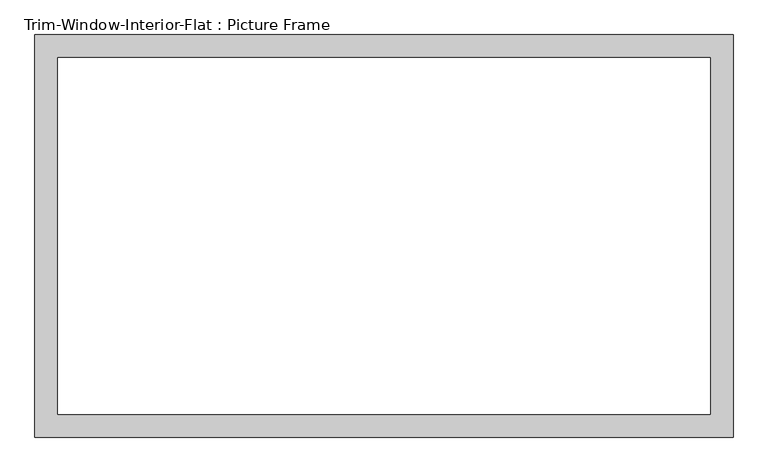
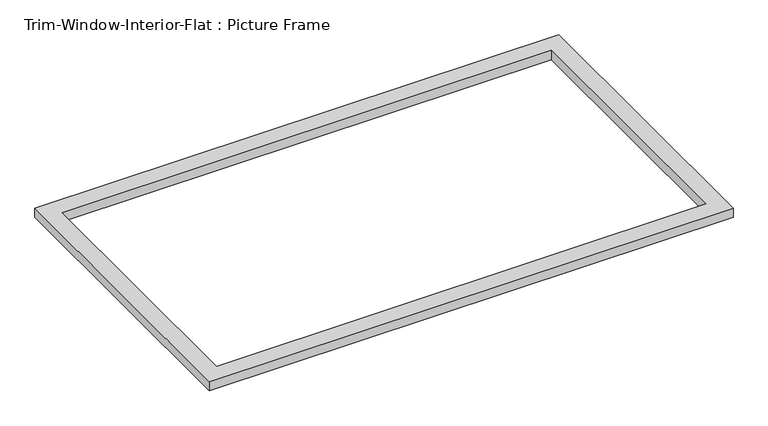
"""IFC4 building model written with IfcOpenShell, lengths in millimetres: proxy geometry, Trim-Window-Interior-Flat : Picture Frame."""

from ifc_helpers import new_model, si_unit, origin, origin_with_axes, place, context, project, spatial, polyline, outline, extrude, source, transform, mapped, element, save


def trim_window_interior_flat_picture_frame_1c33fa8a(model_context):
    return source(origin(), model_context, "Body", "SweptSolid", [
        extrude(outline(polyline([(869.95, 44.45), (869.95, -958.85), (-869.95, -958.85), (-869.95, 44.45), (869.95, 44.45)]), holes=[polyline([(812.8, -12.7), (-812.8, -12.7), (-812.8, -901.7), (812.8, -901.7), (812.8, -12.7)])]), origin_with_axes(), (0.0, 0.0, 1.0), 31.75),
    ])


if __name__ == "__main__":
    model = new_model("IFC4")
    model_context = context("Model", 3, world=origin())
    ifc_project = project(units=[si_unit("LENGTHUNIT", "METRE", prefix="MILLI")], contexts=[model_context])
    site = spatial("IfcSite", under=ifc_project)
    building = spatial("IfcBuilding", under=site)
    placement = place(None, origin())
    trim_window_interior_flat_picture_frame_shape = trim_window_interior_flat_picture_frame_1c33fa8a(model_context)
    element("IfcBuildingElementProxy", 1, Name="Trim-Window-Interior-Flat : Picture Frame", ObjectType="Trim-Window-Interior-Flat : Picture Frame", at=placement, inside=building, context=model_context, shape_type="MappedRepresentation", body=[
        mapped(trim_window_interior_flat_picture_frame_shape, transform((0.0, 0.0, 0.0), x_axis=(1.0, 0.0, 0.0), y_axis=(0.0, 1.0, 0.0), z_axis=(0.0, 0.0, 1.0))),
    ])
    save(model, "model.ifc")

# Revit data of these elements
# Type "Trim-Window-Interior-Flat : Picture Frame"
#   Trim Thickness_Picture Frame = 0' - 1 1/4"
#   Trim Width = 0' - 2 1/4"
#   Trim Thickness_with Sill = 0' - 0 3/4"
#   Sill Thickness = 0' - 1 1/4"
#   Opening Width [instance default] = 2' - 0"
#   Opening Height [instance default] = 3' - 0"
#   Default Elevation = 4' - 0"
#   Sill = no
#   Picture Frame = yes
#   Trim Material [instance default] = none
# Element 1 (IfcBuildingElementProxy, "Trim-Window-Interior-Flat : Picture Frame")
#   Opening Width = 5' - 5"
#   Trim Material = Wood - Stained
#   Materials on its faces: "Wood - Stained"
# Materials
#   "Wood - Stained": class "Wood", colour RGB 224 178 126, transparency 0, Cost = 0
